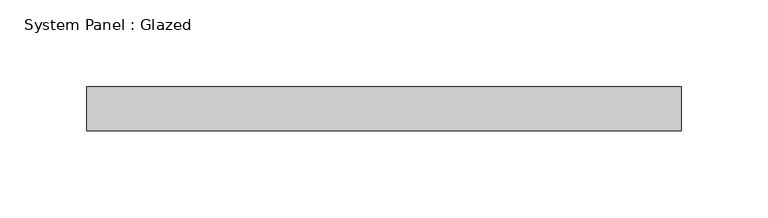
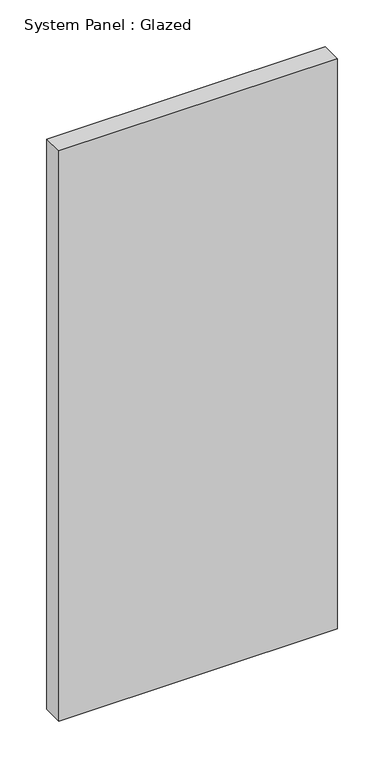
"""IFC4 building model written with IfcOpenShell, lengths in millimetres: plate geometry, System Panel : Glazed."""

from ifc_helpers import new_model, si_unit, origin, origin_with_axes, place, context, project, spatial, polyline, outline, extrude, source, transform, mapped, element, save


def system_panel_glazed_dcf6fd09(model_context):
    return source(origin(), model_context, "Body", "SweptSolid", [
        extrude(outline(polyline([(171.45, 19.05), (-171.45, 19.05), (-171.45, 44.45), (171.45, 44.45), (171.45, 19.05)])), origin_with_axes(), (0.0, 0.0, 1.0), 742.95),
    ])


if __name__ == "__main__":
    model = new_model("IFC4")
    model_context = context("Model", 3, world=origin())
    ifc_project = project(units=[si_unit("LENGTHUNIT", "METRE", prefix="MILLI")], contexts=[model_context])
    site = spatial("IfcSite", under=ifc_project)
    building = spatial("IfcBuilding", under=site)
    placement = place(None, origin())
    system_panel_glazed_shape = system_panel_glazed_dcf6fd09(model_context)
    element("IfcPlate", 1, ObjectType="System Panel : Glazed", at=placement, inside=building, context=model_context, shape_type="MappedRepresentation", body=[
        mapped(system_panel_glazed_shape, transform((0.0, 0.0, 0.0), x_axis=(1.0, 0.0, 0.0), y_axis=(0.0, 1.0, 0.0), z_axis=(0.0, 0.0, 1.0))),
    ])
    save(model, "model.ifc")

# Revit data of these elements
# Type "System Panel : Glazed"
#   Construction Type Id = "GSP4R"
#   Analytic Construction = "1/8 in Pilkington single glazing"
#   Visual Light Transmittance = 0.9
#   Solar Heat Gain Coefficient = 0.86
#   Heat Transfer Coefficient (U) = 1.18115 BTU/(h·ft²·°F)
# Element 1 (IfcPlate, "System Panel : Glazed")
#   Materials on its faces: "Glass"
# Materials
#   "Glass": class "Glass", colour RGB 0 128 192, transparency 0.75, Description = "Soda Lime Glass", Cost = 0
